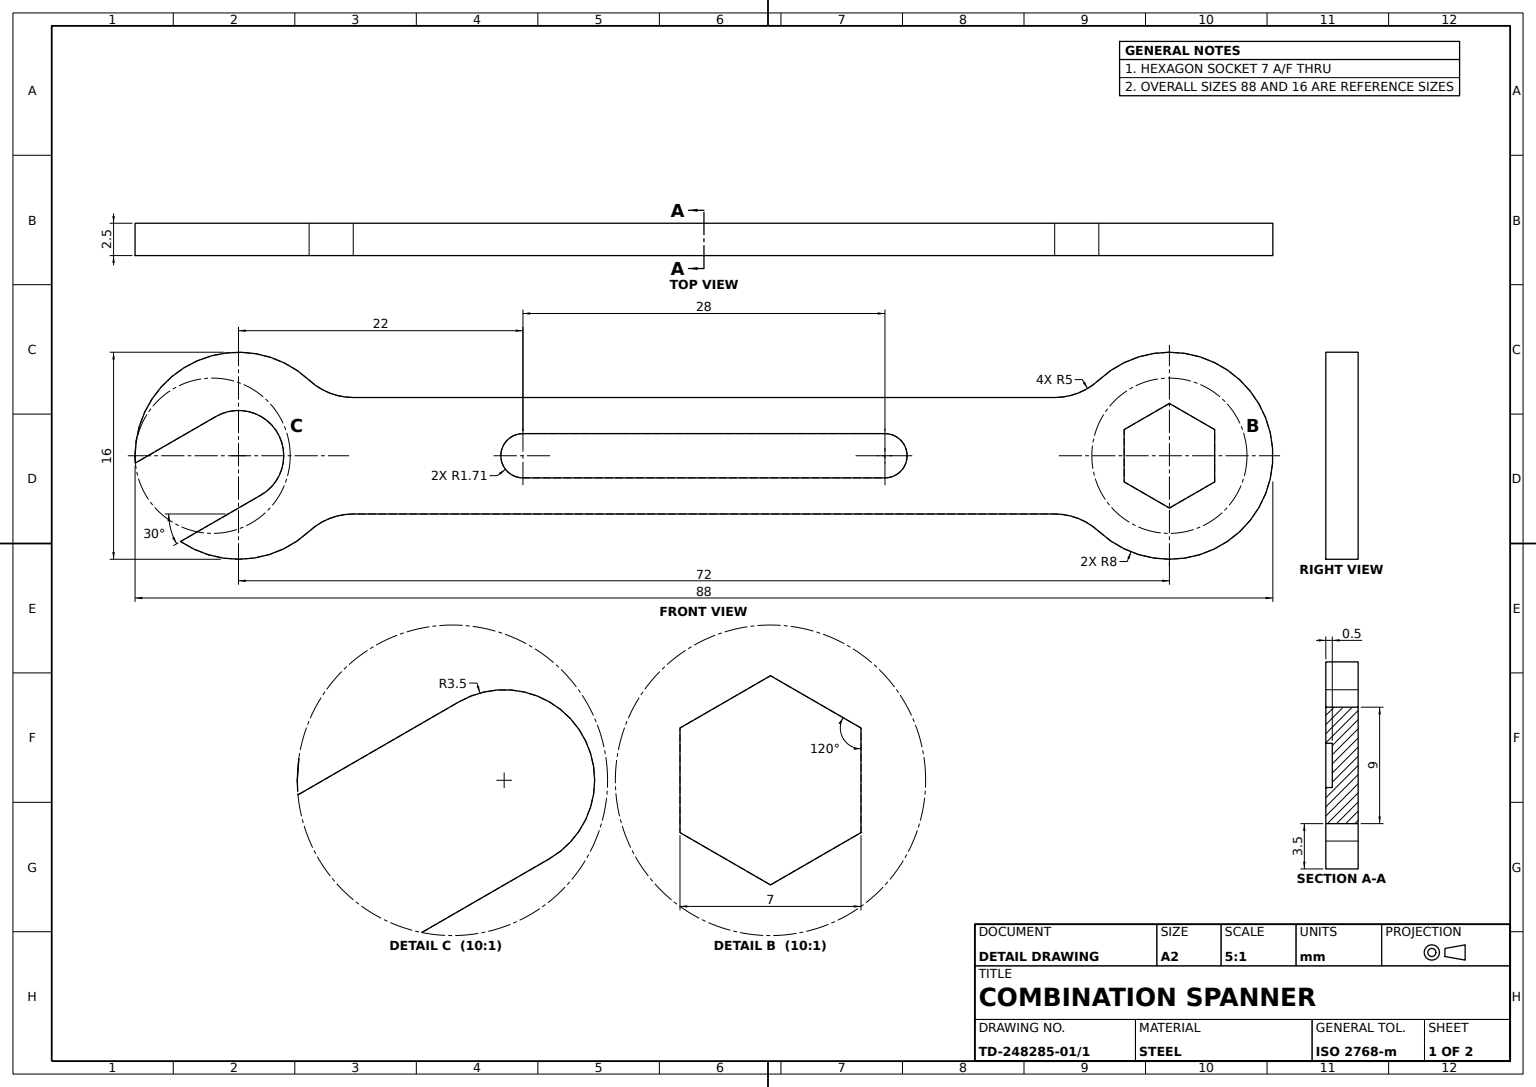
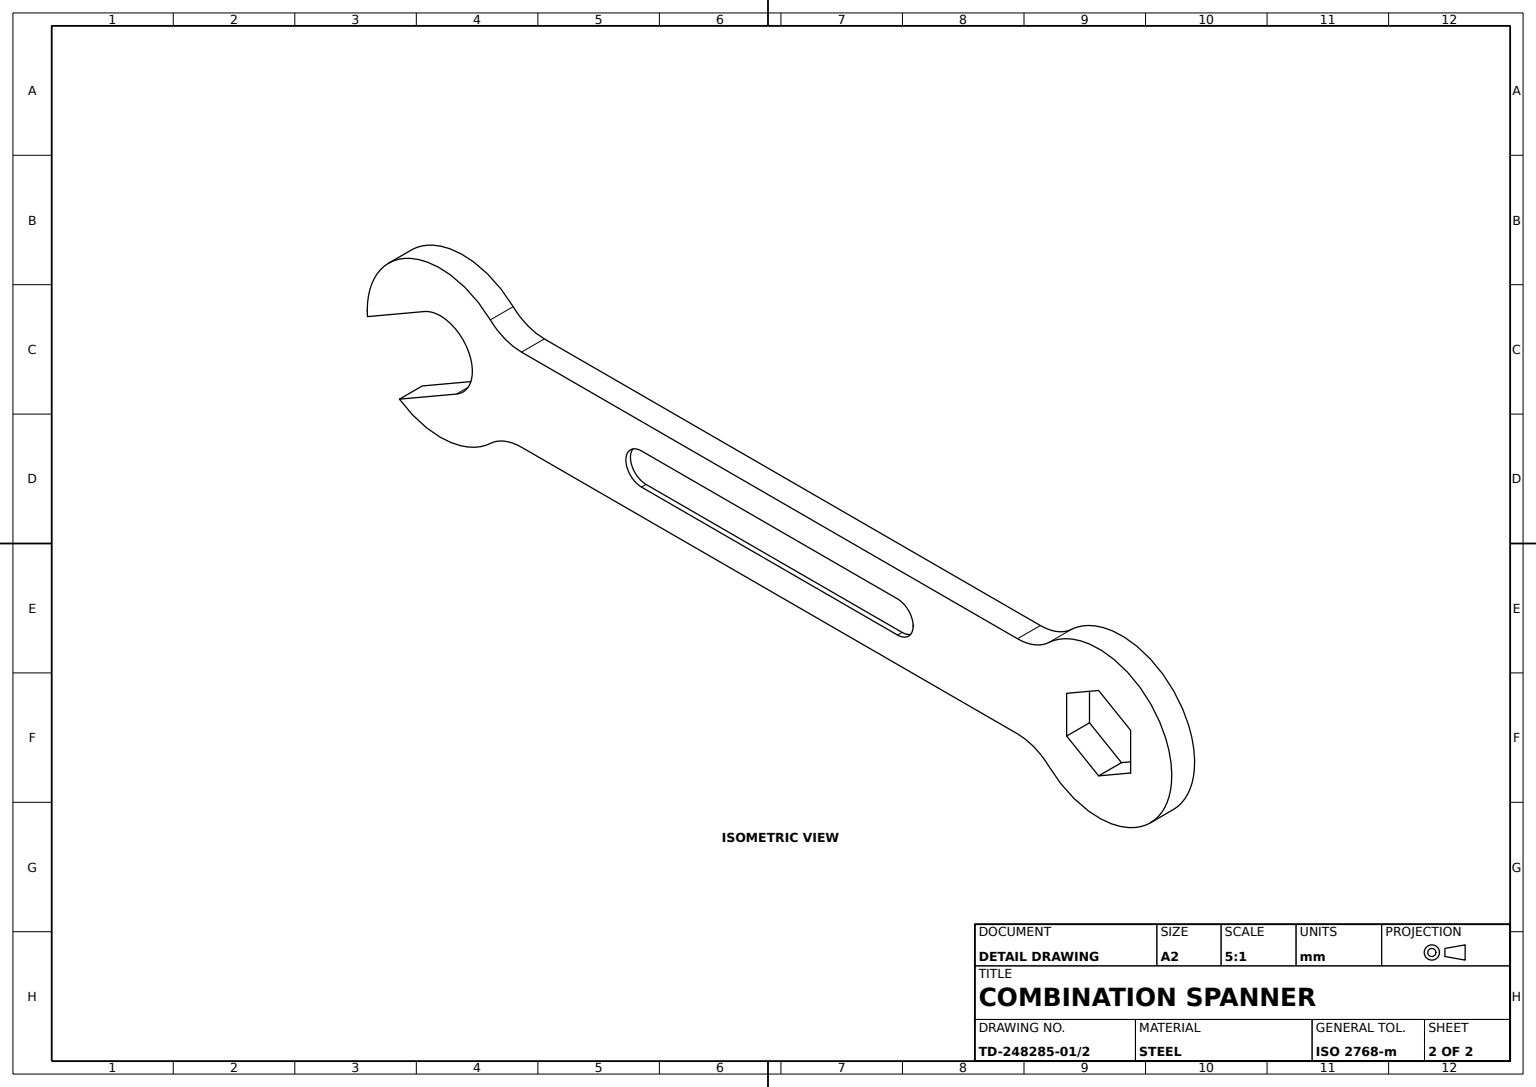
from build123d import *

# Parameters (mm, degrees)
SPANNER_BODY_2_5MM_DEPTH       = 2.5
HANDLE_SLOT_RECESS_0_5MM_DEPTH = 0.5


with BuildPart() as part:
    # Spanner Outline Sketch → Spanner Body 2.5mm (new body)
    with BuildSketch(Plane.XY):
        with BuildLine():
            Line((8.874119675, -4.5), (63.125880325, -4.5))
            ThreePointArc((63.125880325, -4.5), (64.96037879, -4.848697453), (66.539003277, -5.846153846))
            ThreePointArc((66.539003277, -5.846153846), (80, 0), (66.539003277, 5.846153846))
            ThreePointArc((66.539003277, 5.846153846), (64.96037879, 4.848697453), (63.125880325, 4.5))
            Line((63.125880325, 4.5), (8.874119675, 4.5))
            ThreePointArc((8.874119675, 4.5), (7.03962121, 4.848697453), (5.460996723, 5.846153846))
            ThreePointArc((5.460996723, 5.846153846), (-3.444494595, 7.220488694), (-7.979967897, -0.565784729))
            Line((-7.979967897, -0.565784729), (-1.75, 3.031088913))
            ThreePointArc((-1.75, 3.031088913), (3.031088913, 1.75), (1.75, -3.031088913))
            Line((1.75, -3.031088913), (-4.479967897, -6.627962556))
            ThreePointArc((-4.479967897, -6.627962556), (0.627224524, -7.975373935), (5.460996723, -5.846153846))
            ThreePointArc((5.460996723, -5.846153846), (7.03962121, -4.848697453), (8.874119675, -4.5))
        make_face()
        Polygon((75.5, -2.020725942), (75.5, 2.020725942), (72, 4.041451884), (68.5, 2.020725942), (68.5, -2.020725942), (72, -4.041451884), align=None, mode=Mode.SUBTRACT)
    extrude(amount=SPANNER_BODY_2_5MM_DEPTH)

    # Handle Slot Sketch → Handle Slot Recess 0.5mm (cut)
    with BuildSketch(Plane.XY.offset(2.5)):
        with BuildLine():
            Line((22, 1.71110999), (50, 1.71110999))
            ThreePointArc((50, 1.71110999), (51.71110999, 0), (50, -1.71110999))
            Line((50, -1.71110999), (22, -1.71110999))
            ThreePointArc((22, -1.71110999), (20.28889001, 0), (22, 1.71110999))
        make_face()
    extrude(amount=-HANDLE_SLOT_RECESS_0_5MM_DEPTH, mode=Mode.SUBTRACT)


solid = part.part
